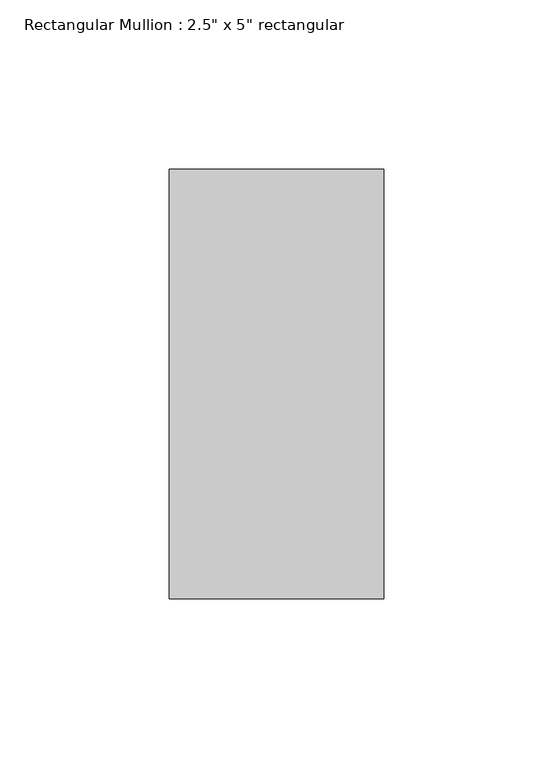
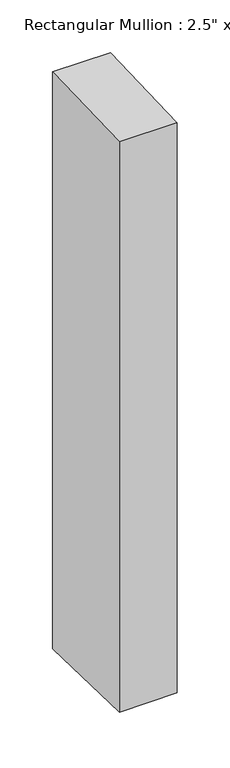
"""IFC4 building model written with IfcOpenShell, lengths in millimetres: member geometry."""

from ifc_helpers import new_model, si_unit, frame, origin, place, context, project, spatial, polyline, outline, extrude, source, transform, mapped, element, save


def member_6fafe7ef(model_context):
    return source(origin(), model_context, "Body", "SweptSolid", [
        extrude(outline(polyline([(-63.5, -2.0787748), (63.5, 2.0787748), (63.5, -667.0795774), (-63.5, -663.1993765), (-63.5, -2.0787748)])), frame((-63.5, 0.0, 0.0), z_axis=(1.0, 0.0, 0.0), x_axis=(0.0, 1.0, 0.0)), (0.0, 0.0, 1.0), 63.5),
    ])


if __name__ == "__main__":
    model = new_model("IFC4")
    model_context = context("Model", 3, world=origin())
    ifc_project = project(units=[si_unit("LENGTHUNIT", "METRE", prefix="MILLI")], contexts=[model_context])
    site = spatial("IfcSite", under=ifc_project)
    building = spatial("IfcBuilding", under=site)
    placement = place(None, origin())
    member_shape = member_6fafe7ef(model_context)
    element("IfcMember", 1, ObjectType="Rectangular Mullion : 2.5\" x 5\" rectangular", at=placement, inside=building, context=model_context, shape_type="MappedRepresentation", body=[
        mapped(member_shape, transform((0.0, 0.0, 0.0), x_axis=(1.0, 0.0, 0.0), y_axis=(0.0, 1.0, 0.0), z_axis=(0.0, 0.0, 1.0))),
    ])
    save(model, "model.ifc")

# Revit data of these elements
# Type "Rectangular Mullion : 2.5\" x 5\" rectangular"
#   built-in parameter 1007304 = 0.416667 (stored number, unit not read)
#   built-in parameter 1007301 = 0.104167 (stored number, unit not read)
#   built-in parameter 1007300 = 0.104167 (stored number, unit not read)
# Element 1 (IfcMember, "Rectangular Mullion : 2.5\" x 5\" rectangular")
#   Materials on its faces: "Aluminum"
# Materials
#   "Aluminum": class "Metal", colour RGB 247 247 247, transparency 0, Description = "Aluminum 6061", Cost = 0
